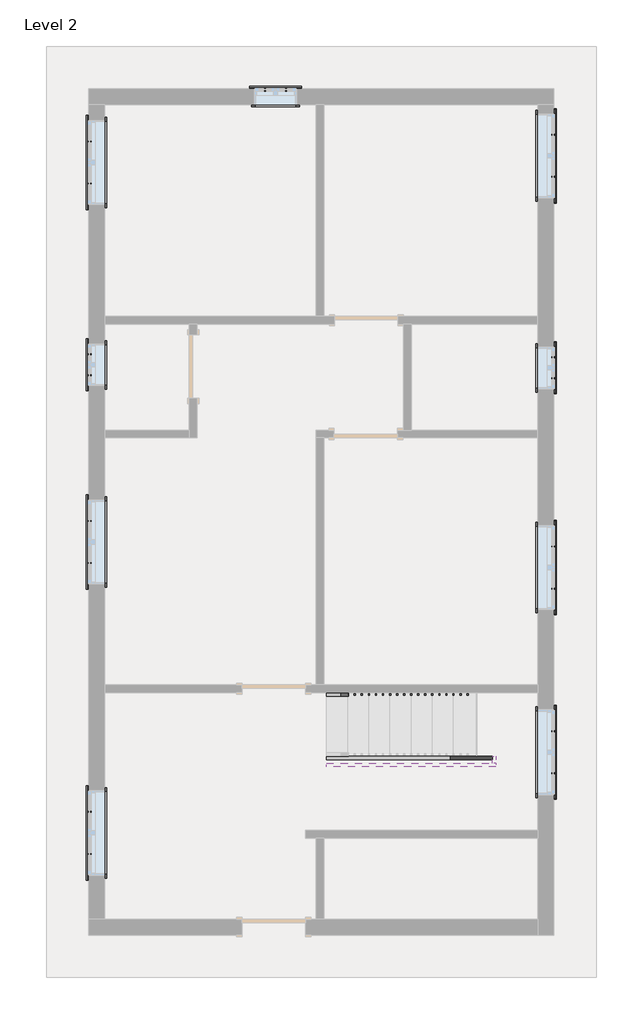
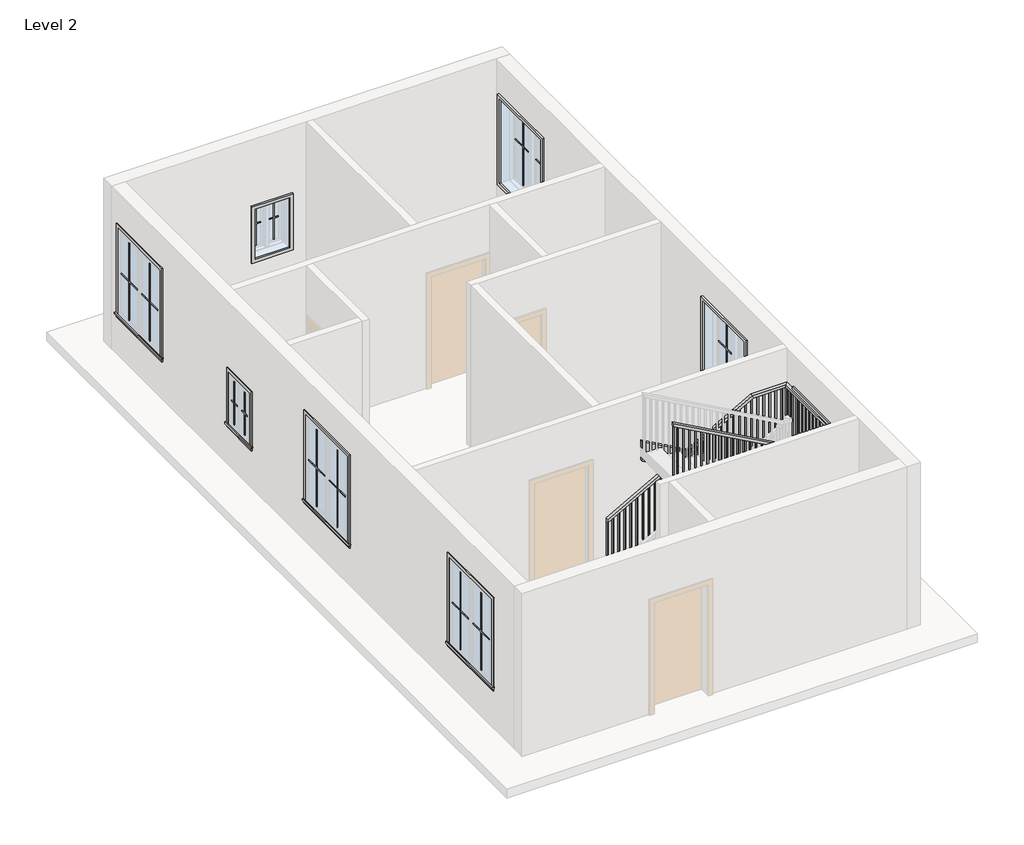
# One storey, part 2 of 2: 36 proxies, 3 members, 1 railing.
"""IFC4 building model written with IfcOpenShell, lengths in millimetres."""

from ifc_helpers import new_model, si_unit, frame, origin, place, context, project, spatial, polyline, outline, extrude, faceted_brep, transform, mapped, element, save
from components import muntin_pattern_2x2_muntin_pattern_2x2_6dad3731, muntin_pattern_2x2_muntin_pattern_2x2_a30a3345, muntin_pattern_2x2_muntin_pattern_2x2_53152e2c, muntin_pattern_2x2_muntin_pattern_2x2_e8f3e573, trim_window_exterior_flat_with_sill_92b9b949, trim_window_exterior_flat_with_sill_a665a915, trim_window_interior_flat_picture_frame_3bb882cf, trim_window_interior_flat_picture_frame_d485c387

model = new_model("IFC4")

# Units and contexts
model_context = context("Model", 3, world=origin())
ifc_project = project(units=[si_unit("LENGTHUNIT", "METRE", prefix="MILLI")], contexts=[model_context])

# Site, building, storey
site = spatial("IfcSite", under=ifc_project)
building = spatial("IfcBuilding", under=site)
storey = spatial("IfcBuildingStorey", under=building, Name="Level 2", Elevation=3048.0)

# Proxies
placement = place(None, origin())
muntin_pattern_2x2_muntin_pattern_2x2_shape = muntin_pattern_2x2_muntin_pattern_2x2_6dad3731(model_context)
element("IfcBuildingElementProxy", 1, Name="Muntin Pattern_2x2 : Muntin Pattern_2x2", ObjectType="Muntin Pattern_2x2 : Muntin Pattern_2x2", at=placement, inside=storey, context=model_context, shape_type="MappedRepresentation", body=[
    mapped(muntin_pattern_2x2_muntin_pattern_2x2_shape, transform((1279.525, 2947.4914062, 4032.25), x_axis=(0.0, 1.0, 0.0), y_axis=(-1.0, 0.0, 0.0), z_axis=(0.0, 0.0, 1.0))),
])
element("IfcBuildingElementProxy", 2, Name="Muntin Pattern_2x2 : Muntin Pattern_2x2", ObjectType="Muntin Pattern_2x2 : Muntin Pattern_2x2", at=placement, inside=storey, context=model_context, shape_type="MappedRepresentation", body=[
    mapped(muntin_pattern_2x2_muntin_pattern_2x2_shape, transform((1279.525, 7138.4914062, 4032.25), x_axis=(0.0, 1.0, 0.0), y_axis=(-1.0, 0.0, 0.0), z_axis=(0.0, 0.0, 1.0))),
])
element("IfcBuildingElementProxy", 3, Name="Muntin Pattern_2x2 : Muntin Pattern_2x2", ObjectType="Muntin Pattern_2x2 : Muntin Pattern_2x2", at=placement, inside=storey, context=model_context, shape_type="MappedRepresentation", body=[
    mapped(muntin_pattern_2x2_muntin_pattern_2x2_shape, transform((1279.525, 12605.8414062, 4032.25), x_axis=(0.0, 1.0, 0.0), y_axis=(-1.0, 0.0, 0.0), z_axis=(0.0, 0.0, 1.0))),
])
element("IfcBuildingElementProxy", 4, Name="Muntin Pattern_2x2 : Muntin Pattern_2x2", ObjectType="Muntin Pattern_2x2 : Muntin Pattern_2x2", at=placement, inside=storey, context=model_context, shape_type="MappedRepresentation", body=[
    mapped(muntin_pattern_2x2_muntin_pattern_2x2_shape, transform((7966.075, 13308.0125, 4032.25), x_axis=(0.0, -1.0, 0.0), y_axis=(1.0, 0.0, 0.0), z_axis=(0.0, 0.0, 1.0))),
])
element("IfcBuildingElementProxy", 5, Name="Muntin Pattern_2x2 : Muntin Pattern_2x2", ObjectType="Muntin Pattern_2x2 : Muntin Pattern_2x2", at=placement, inside=storey, context=model_context, shape_type="MappedRepresentation", body=[
    mapped(muntin_pattern_2x2_muntin_pattern_2x2_shape, transform((7966.075, 7377.1125, 4032.25), x_axis=(0.0, -1.0, 0.0), y_axis=(1.0, 0.0, 0.0), z_axis=(0.0, 0.0, 1.0))),
])
element("IfcBuildingElementProxy", 6, Name="Muntin Pattern_2x2 : Muntin Pattern_2x2", ObjectType="Muntin Pattern_2x2 : Muntin Pattern_2x2", at=placement, inside=storey, context=model_context, shape_type="MappedRepresentation", body=[
    mapped(muntin_pattern_2x2_muntin_pattern_2x2_shape, transform((7966.075, 4716.4625, 4032.25), x_axis=(0.0, -1.0, 0.0), y_axis=(1.0, 0.0, 0.0), z_axis=(0.0, 0.0, 1.0))),
])
muntin_pattern_2x2_muntin_pattern_2x2_2_shape = muntin_pattern_2x2_muntin_pattern_2x2_a30a3345(model_context)
element("IfcBuildingElementProxy", 7, Name="Muntin Pattern_2x2 : Muntin Pattern_2x2", ObjectType="Muntin Pattern_2x2 : Muntin Pattern_2x2", at=placement, inside=storey, context=model_context, shape_type="MappedRepresentation", body=[
    mapped(muntin_pattern_2x2_muntin_pattern_2x2_2_shape, transform((1279.525, 3553.9164063, 4032.25), x_axis=(0.0, -1.0, 0.0), y_axis=(1.0, 0.0, 0.0), z_axis=(0.0, 0.0, 1.0))),
])
element("IfcBuildingElementProxy", 8, Name="Muntin Pattern_2x2 : Muntin Pattern_2x2", ObjectType="Muntin Pattern_2x2 : Muntin Pattern_2x2", at=placement, inside=storey, context=model_context, shape_type="MappedRepresentation", body=[
    mapped(muntin_pattern_2x2_muntin_pattern_2x2_2_shape, transform((1279.525, 7744.9164062, 4032.25), x_axis=(0.0, -1.0, 0.0), y_axis=(1.0, 0.0, 0.0), z_axis=(0.0, 0.0, 1.0))),
])
element("IfcBuildingElementProxy", 9, Name="Muntin Pattern_2x2 : Muntin Pattern_2x2", ObjectType="Muntin Pattern_2x2 : Muntin Pattern_2x2", at=placement, inside=storey, context=model_context, shape_type="MappedRepresentation", body=[
    mapped(muntin_pattern_2x2_muntin_pattern_2x2_2_shape, transform((1279.525, 13212.2664062, 4032.25), x_axis=(0.0, -1.0, 0.0), y_axis=(1.0, 0.0, 0.0), z_axis=(0.0, 0.0, 1.0))),
])
element("IfcBuildingElementProxy", 10, Name="Muntin Pattern_2x2 : Muntin Pattern_2x2", ObjectType="Muntin Pattern_2x2 : Muntin Pattern_2x2", at=placement, inside=storey, context=model_context, shape_type="MappedRepresentation", body=[
    mapped(muntin_pattern_2x2_muntin_pattern_2x2_2_shape, transform((7966.075, 12701.5875, 4032.25), x_axis=(0.0, 1.0, 0.0), y_axis=(-1.0, 0.0, 0.0), z_axis=(0.0, 0.0, 1.0))),
])
element("IfcBuildingElementProxy", 11, Name="Muntin Pattern_2x2 : Muntin Pattern_2x2", ObjectType="Muntin Pattern_2x2 : Muntin Pattern_2x2", at=placement, inside=storey, context=model_context, shape_type="MappedRepresentation", body=[
    mapped(muntin_pattern_2x2_muntin_pattern_2x2_2_shape, transform((7966.075, 6770.6875, 4032.25), x_axis=(0.0, 1.0, 0.0), y_axis=(-1.0, 0.0, 0.0), z_axis=(0.0, 0.0, 1.0))),
])
element("IfcBuildingElementProxy", 12, Name="Muntin Pattern_2x2 : Muntin Pattern_2x2", ObjectType="Muntin Pattern_2x2 : Muntin Pattern_2x2", at=placement, inside=storey, context=model_context, shape_type="MappedRepresentation", body=[
    mapped(muntin_pattern_2x2_muntin_pattern_2x2_2_shape, transform((7966.075, 4110.0375, 4032.25), x_axis=(0.0, 1.0, 0.0), y_axis=(-1.0, 0.0, 0.0), z_axis=(0.0, 0.0, 1.0))),
])
muntin_pattern_2x2_muntin_pattern_2x2_3_shape = muntin_pattern_2x2_muntin_pattern_2x2_53152e2c(model_context)
element("IfcBuildingElementProxy", 13, Name="Muntin Pattern_2x2 : Muntin Pattern_2x2", ObjectType="Muntin Pattern_2x2 : Muntin Pattern_2x2", at=placement, inside=storey, context=model_context, shape_type="MappedRepresentation", body=[
    mapped(muntin_pattern_2x2_muntin_pattern_2x2_3_shape, transform((3811.5875, 13960.475, 4032.25), x_axis=(1.0, 0.0, 0.0), y_axis=(0.0, 1.0, 0.0), z_axis=(0.0, 0.0, 1.0))),
])
element("IfcBuildingElementProxy", 14, Name="Muntin Pattern_2x2 : Muntin Pattern_2x2", ObjectType="Muntin Pattern_2x2 : Muntin Pattern_2x2", at=placement, inside=storey, context=model_context, shape_type="MappedRepresentation", body=[
    mapped(muntin_pattern_2x2_muntin_pattern_2x2_3_shape, transform((7966.075, 10101.2625, 4032.25), x_axis=(0.0, -1.0, 0.0), y_axis=(1.0, 0.0, 0.0), z_axis=(0.0, 0.0, 1.0))),
])
element("IfcBuildingElementProxy", 15, Name="Muntin Pattern_2x2 : Muntin Pattern_2x2", ObjectType="Muntin Pattern_2x2 : Muntin Pattern_2x2", at=placement, inside=storey, context=model_context, shape_type="MappedRepresentation", body=[
    mapped(muntin_pattern_2x2_muntin_pattern_2x2_3_shape, transform((1279.525, 9843.5914062, 4032.25), x_axis=(0.0, 1.0, 0.0), y_axis=(-1.0, 0.0, 0.0), z_axis=(0.0, 0.0, 1.0))),
])
muntin_pattern_2x2_muntin_pattern_2x2_4_shape = muntin_pattern_2x2_muntin_pattern_2x2_e8f3e573(model_context)
element("IfcBuildingElementProxy", 16, Name="Muntin Pattern_2x2 : Muntin Pattern_2x2", ObjectType="Muntin Pattern_2x2 : Muntin Pattern_2x2", at=placement, inside=storey, context=model_context, shape_type="MappedRepresentation", body=[
    mapped(muntin_pattern_2x2_muntin_pattern_2x2_4_shape, transform((4113.2125, 13960.475, 4032.25), x_axis=(-1.0, 0.0, 0.0), y_axis=(0.0, -1.0, 0.0), z_axis=(0.0, 0.0, 1.0))),
])
element("IfcBuildingElementProxy", 17, Name="Muntin Pattern_2x2 : Muntin Pattern_2x2", ObjectType="Muntin Pattern_2x2 : Muntin Pattern_2x2", at=placement, inside=storey, context=model_context, shape_type="MappedRepresentation", body=[
    mapped(muntin_pattern_2x2_muntin_pattern_2x2_4_shape, transform((7966.075, 9799.6375, 4032.25), x_axis=(0.0, 1.0, 0.0), y_axis=(-1.0, 0.0, 0.0), z_axis=(0.0, 0.0, 1.0))),
])
element("IfcBuildingElementProxy", 18, Name="Muntin Pattern_2x2 : Muntin Pattern_2x2", ObjectType="Muntin Pattern_2x2 : Muntin Pattern_2x2", at=placement, inside=storey, context=model_context, shape_type="MappedRepresentation", body=[
    mapped(muntin_pattern_2x2_muntin_pattern_2x2_4_shape, transform((1279.525, 10145.2164062, 4032.25), x_axis=(0.0, -1.0, 0.0), y_axis=(1.0, 0.0, 0.0), z_axis=(0.0, 0.0, 1.0))),
])
trim_window_exterior_flat_with_sill_shape = trim_window_exterior_flat_with_sill_92b9b949(model_context)
element("IfcBuildingElementProxy", 19, Name="Trim-Window-Exterior-Flat : with Sill", ObjectType="Trim-Window-Exterior-Flat : with Sill", at=placement, inside=storey, context=model_context, shape_type="MappedRepresentation", body=[
    mapped(trim_window_exterior_flat_with_sill_shape, transform((1270.0, 3250.7039063, 5486.4), x_axis=(0.0, -1.0, 0.0), y_axis=(0.0, 0.0, 1.0), z_axis=(-1.0, 0.0, 0.0))),
])
element("IfcBuildingElementProxy", 20, Name="Trim-Window-Exterior-Flat : with Sill", ObjectType="Trim-Window-Exterior-Flat : with Sill", at=placement, inside=storey, context=model_context, shape_type="MappedRepresentation", body=[
    mapped(trim_window_exterior_flat_with_sill_shape, transform((1270.0, 7441.7039063, 5486.4), x_axis=(0.0, -1.0, 0.0), y_axis=(0.0, 0.0, 1.0), z_axis=(-1.0, 0.0, 0.0))),
])
element("IfcBuildingElementProxy", 21, Name="Trim-Window-Exterior-Flat : with Sill", ObjectType="Trim-Window-Exterior-Flat : with Sill", at=placement, inside=storey, context=model_context, shape_type="MappedRepresentation", body=[
    mapped(trim_window_exterior_flat_with_sill_shape, transform((1270.0, 12909.0539063, 5486.4), x_axis=(0.0, -1.0, 0.0), y_axis=(0.0, 0.0, 1.0), z_axis=(-1.0, 0.0, 0.0))),
])
element("IfcBuildingElementProxy", 22, Name="Trim-Window-Exterior-Flat : with Sill", ObjectType="Trim-Window-Exterior-Flat : with Sill", at=placement, inside=storey, context=model_context, shape_type="MappedRepresentation", body=[
    mapped(trim_window_exterior_flat_with_sill_shape, transform((7975.6, 13004.8, 5486.4), x_axis=(0.0, 1.0, 0.0), y_axis=(0.0, 0.0, 1.0), z_axis=(1.0, 0.0, 0.0))),
])
element("IfcBuildingElementProxy", 23, Name="Trim-Window-Exterior-Flat : with Sill", ObjectType="Trim-Window-Exterior-Flat : with Sill", at=placement, inside=storey, context=model_context, shape_type="MappedRepresentation", body=[
    mapped(trim_window_exterior_flat_with_sill_shape, transform((7975.6, 7073.9, 5486.4), x_axis=(0.0, 1.0, 0.0), y_axis=(0.0, 0.0, 1.0), z_axis=(1.0, 0.0, 0.0))),
])
element("IfcBuildingElementProxy", 24, Name="Trim-Window-Exterior-Flat : with Sill", ObjectType="Trim-Window-Exterior-Flat : with Sill", at=placement, inside=storey, context=model_context, shape_type="MappedRepresentation", body=[
    mapped(trim_window_exterior_flat_with_sill_shape, transform((7975.6, 4413.25, 5486.4), x_axis=(0.0, 1.0, 0.0), y_axis=(0.0, 0.0, 1.0), z_axis=(1.0, 0.0, 0.0))),
])
trim_window_exterior_flat_with_sill_2_shape = trim_window_exterior_flat_with_sill_a665a915(model_context)
element("IfcBuildingElementProxy", 25, Name="Trim-Window-Exterior-Flat : with Sill", ObjectType="Trim-Window-Exterior-Flat : with Sill", at=placement, inside=storey, context=model_context, shape_type="MappedRepresentation", body=[
    mapped(trim_window_exterior_flat_with_sill_2_shape, transform((3962.4, 13970.0, 4876.8), x_axis=(-1.0, 0.0, 0.0), y_axis=(0.0, 0.0, 1.0), z_axis=(0.0, 1.0, 0.0))),
])
element("IfcBuildingElementProxy", 26, Name="Trim-Window-Exterior-Flat : with Sill", ObjectType="Trim-Window-Exterior-Flat : with Sill", at=placement, inside=storey, context=model_context, shape_type="MappedRepresentation", body=[
    mapped(trim_window_exterior_flat_with_sill_2_shape, transform((7975.6, 9950.45, 4876.8), x_axis=(0.0, 1.0, 0.0), y_axis=(0.0, 0.0, 1.0), z_axis=(1.0, 0.0, 0.0))),
])
element("IfcBuildingElementProxy", 27, Name="Trim-Window-Exterior-Flat : with Sill", ObjectType="Trim-Window-Exterior-Flat : with Sill", at=placement, inside=storey, context=model_context, shape_type="MappedRepresentation", body=[
    mapped(trim_window_exterior_flat_with_sill_2_shape, transform((1270.0, 9994.4039062, 4876.8), x_axis=(0.0, -1.0, 0.0), y_axis=(0.0, 0.0, 1.0), z_axis=(-1.0, 0.0, 0.0))),
])
trim_window_interior_flat_picture_frame_shape = trim_window_interior_flat_picture_frame_3bb882cf(model_context)
element("IfcBuildingElementProxy", 28, Name="Trim-Window-Interior-Flat : Picture Frame", ObjectType="Trim-Window-Interior-Flat : Picture Frame", at=placement, inside=storey, context=model_context, shape_type="MappedRepresentation", body=[
    mapped(trim_window_interior_flat_picture_frame_shape, transform((1498.6, 3250.7039063, 5486.4), x_axis=(0.0, 1.0, 0.0), y_axis=(0.0, 0.0, 1.0), z_axis=(1.0, 0.0, 0.0))),
])
element("IfcBuildingElementProxy", 29, Name="Trim-Window-Interior-Flat : Picture Frame", ObjectType="Trim-Window-Interior-Flat : Picture Frame", at=placement, inside=storey, context=model_context, shape_type="MappedRepresentation", body=[
    mapped(trim_window_interior_flat_picture_frame_shape, transform((1498.6, 7441.7039062, 5486.4), x_axis=(0.0, 1.0, 0.0), y_axis=(0.0, 0.0, 1.0), z_axis=(1.0, 0.0, 0.0))),
])
element("IfcBuildingElementProxy", 30, Name="Trim-Window-Interior-Flat : Picture Frame", ObjectType="Trim-Window-Interior-Flat : Picture Frame", at=placement, inside=storey, context=model_context, shape_type="MappedRepresentation", body=[
    mapped(trim_window_interior_flat_picture_frame_shape, transform((1498.6, 12909.0539062, 5486.4), x_axis=(0.0, 1.0, 0.0), y_axis=(0.0, 0.0, 1.0), z_axis=(1.0, 0.0, 0.0))),
])
element("IfcBuildingElementProxy", 31, Name="Trim-Window-Interior-Flat : Picture Frame", ObjectType="Trim-Window-Interior-Flat : Picture Frame", at=placement, inside=storey, context=model_context, shape_type="MappedRepresentation", body=[
    mapped(trim_window_interior_flat_picture_frame_shape, transform((7747.0, 13004.8, 5486.4), x_axis=(0.0, -1.0, 0.0), y_axis=(0.0, 0.0, 1.0), z_axis=(-1.0, 0.0, 0.0))),
])
element("IfcBuildingElementProxy", 32, Name="Trim-Window-Interior-Flat : Picture Frame", ObjectType="Trim-Window-Interior-Flat : Picture Frame", at=placement, inside=storey, context=model_context, shape_type="MappedRepresentation", body=[
    mapped(trim_window_interior_flat_picture_frame_shape, transform((7747.0, 7073.9, 5486.4), x_axis=(0.0, -1.0, 0.0), y_axis=(0.0, 0.0, 1.0), z_axis=(-1.0, 0.0, 0.0))),
])
element("IfcBuildingElementProxy", 33, Name="Trim-Window-Interior-Flat : Picture Frame", ObjectType="Trim-Window-Interior-Flat : Picture Frame", at=placement, inside=storey, context=model_context, shape_type="MappedRepresentation", body=[
    mapped(trim_window_interior_flat_picture_frame_shape, transform((7747.0, 4413.25, 5486.4), x_axis=(0.0, -1.0, 0.0), y_axis=(0.0, 0.0, 1.0), z_axis=(-1.0, 0.0, 0.0))),
])
trim_window_interior_flat_picture_frame_2_shape = trim_window_interior_flat_picture_frame_d485c387(model_context)
element("IfcBuildingElementProxy", 34, Name="Trim-Window-Interior-Flat : Picture Frame", ObjectType="Trim-Window-Interior-Flat : Picture Frame", at=placement, inside=storey, context=model_context, shape_type="MappedRepresentation", body=[
    mapped(trim_window_interior_flat_picture_frame_2_shape, transform((3962.4, 13741.4, 4876.8), x_axis=(1.0, 0.0, 0.0), y_axis=(0.0, 0.0, 1.0), z_axis=(0.0, -1.0, 0.0))),
])
element("IfcBuildingElementProxy", 35, Name="Trim-Window-Interior-Flat : Picture Frame", ObjectType="Trim-Window-Interior-Flat : Picture Frame", at=placement, inside=storey, context=model_context, shape_type="MappedRepresentation", body=[
    mapped(trim_window_interior_flat_picture_frame_2_shape, transform((7747.0, 9950.45, 4876.8), x_axis=(0.0, -1.0, 0.0), y_axis=(0.0, 0.0, 1.0), z_axis=(-1.0, 0.0, 0.0))),
])
element("IfcBuildingElementProxy", 36, Name="Trim-Window-Interior-Flat : Picture Frame", ObjectType="Trim-Window-Interior-Flat : Picture Frame", at=placement, inside=storey, context=model_context, shape_type="MappedRepresentation", body=[
    mapped(trim_window_interior_flat_picture_frame_2_shape, transform((1498.6, 9994.4039062, 4876.8), x_axis=(0.0, 1.0, 0.0), y_axis=(0.0, 0.0, 1.0), z_axis=(1.0, 0.0, 0.0))),
])

# Members
element("IfcMember", 37, ObjectType="Stringer - 2\" Width", at=placement, inside=storey, context=model_context, shape_type="SweptSolid", body=[
    extrude(outline(polyline([(3255.5983948, 4699.0), (3048.0, 4699.0), (3048.0, 4952.9445028), (4233.3641651, 7086.6), (4582.0428392, 7086.6), (3255.5983948, 4699.0)])), frame((0.0, 4305.3, 0.0), z_axis=(0.0, 1.0, 0.0), x_axis=(0.0, 0.0, 1.0)), (0.0, 0.0, 1.0), 50.8),
])
element("IfcMember", 38, ObjectType="Stringer - 2\" Width", at=placement, inside=storey, context=model_context, shape_type="SweptSolid", body=[
    extrude(outline(polyline([(7086.6, 4356.1), (7137.4, 4356.1), (7137.4, 4254.5), (7086.6, 4254.5), (7086.6, 4356.1)])), frame((0.0, 0.0, 4343.4), z_axis=(0.0, 0.0, 1.0), x_axis=(1.0, 0.0, 0.0)), (0.0, 0.0, 1.0), 304.8),
])
element("IfcMember", 39, ObjectType="Stringer - 2\" Width", at=placement, inside=storey, context=model_context, shape_type="SweptSolid", body=[
    extrude(outline(polyline([(4430.9197207, 7137.4), (4779.5983948, 7137.4), (6134.2650614, 4699.0), (5785.5863873, 4699.0), (4430.9197207, 7137.4)])), frame((0.0, 4203.7, 0.0), z_axis=(0.0, 1.0, 0.0), x_axis=(0.0, 0.0, 1.0)), (0.0, 0.0, 1.0), 50.8),
])

# Railing
element("IfcRailing", 40, ObjectType="Handrail - Rectangular", at=placement, inside=storey, context=model_context, shape_type="SolidModel", body=[
    faceted_brep([(4699.0, 5270.5, 4131.7333333), (4699.0, 5270.5, 4073.620221), (4699.0, 5219.7, 4073.620221), (4699.0, 5219.7, 4131.7333333), (7137.4, 5270.5, 5486.4), (7150.5636022, 5270.5, 5435.6), (7150.5636022, 5219.7, 5435.6), (7137.4, 5219.7, 5486.4), (7747.0, 5270.5, 5486.4), (7747.0, 5270.5, 5435.6), (7696.2, 5219.7, 5435.6), (7696.2, 5219.7, 5486.4), (7747.0, 3289.3, 5486.4), (7747.0, 3289.3, 5435.6), (7696.2, 3340.1, 5435.6), (7696.2, 3340.1, 5486.4), (7442.2, 3289.3, 5486.4), (7429.0363978, 3289.3, 5435.6), (7429.0363978, 3340.1, 5435.6), (7442.2, 3340.1, 5486.4), (4699.0, 3289.3, 7010.4), (4699.0, 3340.1, 7010.4), (4699.0, 3340.1, 6952.2868876), (4699.0, 3289.3, 6952.2868876)], [[[0, 1, 2, 3]], [[1, 0, 4, 5]], [[2, 1, 5, 6]], [[3, 2, 6, 7]], [[0, 3, 7, 4]], [[5, 4, 8, 9]], [[6, 5, 9, 10]], [[7, 6, 10, 11]], [[4, 7, 11, 8]], [[9, 8, 12, 13]], [[10, 9, 13, 14]], [[11, 10, 14, 15]], [[8, 11, 15, 12]], [[13, 12, 16, 17]], [[14, 13, 17, 18]], [[15, 14, 18, 19]], [[12, 15, 19, 16]], [[20, 21, 22, 23]], [[17, 16, 20, 23]], [[18, 17, 23, 22]], [[19, 18, 22, 21]], [[16, 19, 21, 20]]]),
    extrude(outline(polyline([(6915.245221, 4765.675), (5926.6666667, 4765.675), (5926.6666667, 4784.725), (6904.6618876, 4784.725), (6915.245221, 4765.675)])), frame((0.0, 3305.175, 0.0), z_axis=(0.0, 1.0, 0.0), x_axis=(0.0, 0.0, 1.0)), (0.0, 0.0, 1.0), 19.05),
    extrude(outline(polyline([(6858.8007765, 4867.275), (5926.6666667, 4867.275), (5926.6666667, 4886.325), (6848.2174432, 4886.325), (6858.8007765, 4867.275)])), frame((0.0, 3305.175, 0.0), z_axis=(0.0, 1.0, 0.0), x_axis=(0.0, 0.0, 1.0)), (0.0, 0.0, 1.0), 19.05),
    extrude(outline(polyline([(6802.3563321, 4968.875), (5926.6666667, 4968.875), (5926.6666667, 4987.925), (6791.7729988, 4987.925), (6802.3563321, 4968.875)])), frame((0.0, 3305.175, 0.0), z_axis=(0.0, 1.0, 0.0), x_axis=(0.0, 0.0, 1.0)), (0.0, 0.0, 1.0), 19.05),
    extrude(outline(polyline([(6745.9118876, 5070.475), (5757.3333333, 5070.475), (5757.3333333, 5089.525), (6735.3285543, 5089.525), (6745.9118876, 5070.475)])), frame((0.0, 3305.175, 0.0), z_axis=(0.0, 1.0, 0.0), x_axis=(0.0, 0.0, 1.0)), (0.0, 0.0, 1.0), 19.05),
    extrude(outline(polyline([(6689.4674432, 5172.075), (5757.3333333, 5172.075), (5757.3333333, 5191.125), (6678.8841099, 5191.125), (6689.4674432, 5172.075)])), frame((0.0, 3305.175, 0.0), z_axis=(0.0, 1.0, 0.0), x_axis=(0.0, 0.0, 1.0)), (0.0, 0.0, 1.0), 19.05),
    extrude(outline(polyline([(6633.0229988, 5273.675), (5757.3333333, 5273.675), (5757.3333333, 5292.725), (6622.4396654, 5292.725), (6633.0229988, 5273.675)])), frame((0.0, 3305.175, 0.0), z_axis=(0.0, 1.0, 0.0), x_axis=(0.0, 0.0, 1.0)), (0.0, 0.0, 1.0), 19.05),
    extrude(outline(polyline([(6576.5785543, 5375.275), (5588.0, 5375.275), (5588.0, 5394.325), (6565.995221, 5394.325), (6576.5785543, 5375.275)])), frame((0.0, 3305.175, 0.0), z_axis=(0.0, 1.0, 0.0), x_axis=(0.0, 0.0, 1.0)), (0.0, 0.0, 1.0), 19.05),
    extrude(outline(polyline([(6520.1341099, 5476.875), (5588.0, 5476.875), (5588.0, 5495.925), (6509.5507765, 5495.925), (6520.1341099, 5476.875)])), frame((0.0, 3305.175, 0.0), z_axis=(0.0, 1.0, 0.0), x_axis=(0.0, 0.0, 1.0)), (0.0, 0.0, 1.0), 19.05),
    extrude(outline(polyline([(6463.6896654, 5578.475), (5588.0, 5578.475), (5588.0, 5597.525), (6453.1063321, 5597.525), (6463.6896654, 5578.475)])), frame((0.0, 3305.175, 0.0), z_axis=(0.0, 1.0, 0.0), x_axis=(0.0, 0.0, 1.0)), (0.0, 0.0, 1.0), 19.05),
    extrude(outline(polyline([(6407.245221, 5680.075), (5418.6666667, 5680.075), (5418.6666667, 5699.125), (6396.6618876, 5699.125), (6407.245221, 5680.075)])), frame((0.0, 3305.175, 0.0), z_axis=(0.0, 1.0, 0.0), x_axis=(0.0, 0.0, 1.0)), (0.0, 0.0, 1.0), 19.05),
    extrude(outline(polyline([(6350.8007765, 5781.675), (5418.6666667, 5781.675), (5418.6666667, 5800.725), (6340.2174432, 5800.725), (6350.8007765, 5781.675)])), frame((0.0, 3305.175, 0.0), z_axis=(0.0, 1.0, 0.0), x_axis=(0.0, 0.0, 1.0)), (0.0, 0.0, 1.0), 19.05),
    extrude(outline(polyline([(6294.3563321, 5883.275), (5418.6666667, 5883.275), (5418.6666667, 5902.325), (6283.7729988, 5902.325), (6294.3563321, 5883.275)])), frame((0.0, 3305.175, 0.0), z_axis=(0.0, 1.0, 0.0), x_axis=(0.0, 0.0, 1.0)), (0.0, 0.0, 1.0), 19.05),
    extrude(outline(polyline([(6237.9118876, 5984.875), (5249.3333333, 5984.875), (5249.3333333, 6003.925), (6227.3285543, 6003.925), (6237.9118876, 5984.875)])), frame((0.0, 3305.175, 0.0), z_axis=(0.0, 1.0, 0.0), x_axis=(0.0, 0.0, 1.0)), (0.0, 0.0, 1.0), 19.05),
    extrude(outline(polyline([(6181.4674432, 6086.475), (5249.3333333, 6086.475), (5249.3333333, 6105.525), (6170.8841099, 6105.525), (6181.4674432, 6086.475)])), frame((0.0, 3305.175, 0.0), z_axis=(0.0, 1.0, 0.0), x_axis=(0.0, 0.0, 1.0)), (0.0, 0.0, 1.0), 19.05),
    extrude(outline(polyline([(6125.0229988, 6188.075), (5249.3333333, 6188.075), (5249.3333333, 6207.125), (6114.4396654, 6207.125), (6125.0229988, 6188.075)])), frame((0.0, 3305.175, 0.0), z_axis=(0.0, 1.0, 0.0), x_axis=(0.0, 0.0, 1.0)), (0.0, 0.0, 1.0), 19.05),
    extrude(outline(polyline([(6068.5785543, 6289.675), (5080.0, 6289.675), (5080.0, 6308.725), (6057.995221, 6308.725), (6068.5785543, 6289.675)])), frame((0.0, 3305.175, 0.0), z_axis=(0.0, 1.0, 0.0), x_axis=(0.0, 0.0, 1.0)), (0.0, 0.0, 1.0), 19.05),
    extrude(outline(polyline([(6012.1341099, 6391.275), (5080.0, 6391.275), (5080.0, 6410.325), (6001.5507765, 6410.325), (6012.1341099, 6391.275)])), frame((0.0, 3305.175, 0.0), z_axis=(0.0, 1.0, 0.0), x_axis=(0.0, 0.0, 1.0)), (0.0, 0.0, 1.0), 19.05),
    extrude(outline(polyline([(5955.6896654, 6492.875), (5080.0, 6492.875), (5080.0, 6511.925), (5945.1063321, 6511.925), (5955.6896654, 6492.875)])), frame((0.0, 3305.175, 0.0), z_axis=(0.0, 1.0, 0.0), x_axis=(0.0, 0.0, 1.0)), (0.0, 0.0, 1.0), 19.05),
    extrude(outline(polyline([(5899.245221, 6594.475), (4910.6666667, 6594.475), (4910.6666667, 6613.525), (5888.6618876, 6613.525), (5899.245221, 6594.475)])), frame((0.0, 3305.175, 0.0), z_axis=(0.0, 1.0, 0.0), x_axis=(0.0, 0.0, 1.0)), (0.0, 0.0, 1.0), 19.05),
    extrude(outline(polyline([(5842.8007765, 6696.075), (4910.6666667, 6696.075), (4910.6666667, 6715.125), (5832.2174432, 6715.125), (5842.8007765, 6696.075)])), frame((0.0, 3305.175, 0.0), z_axis=(0.0, 1.0, 0.0), x_axis=(0.0, 0.0, 1.0)), (0.0, 0.0, 1.0), 19.05),
    extrude(outline(polyline([(5786.3563321, 6797.675), (4910.6666667, 6797.675), (4910.6666667, 6816.725), (5775.7729988, 6816.725), (5786.3563321, 6797.675)])), frame((0.0, 3305.175, 0.0), z_axis=(0.0, 1.0, 0.0), x_axis=(0.0, 0.0, 1.0)), (0.0, 0.0, 1.0), 19.05),
    extrude(outline(polyline([(5729.9118876, 6899.275), (4741.3333333, 6899.275), (4741.3333333, 6918.325), (5719.3285543, 6918.325), (5729.9118876, 6899.275)])), frame((0.0, 3305.175, 0.0), z_axis=(0.0, 1.0, 0.0), x_axis=(0.0, 0.0, 1.0)), (0.0, 0.0, 1.0), 19.05),
    extrude(outline(polyline([(5673.4674432, 7000.875), (4741.3333333, 7000.875), (4741.3333333, 7019.925), (5662.8841099, 7019.925), (5673.4674432, 7000.875)])), frame((0.0, 3305.175, 0.0), z_axis=(0.0, 1.0, 0.0), x_axis=(0.0, 0.0, 1.0)), (0.0, 0.0, 1.0), 19.05),
    extrude(outline(polyline([(5617.0229988, 7102.475), (4741.3333333, 7102.475), (4741.3333333, 7121.525), (5606.4396654, 7121.525), (5617.0229988, 7102.475)])), frame((0.0, 3305.175, 0.0), z_axis=(0.0, 1.0, 0.0), x_axis=(0.0, 0.0, 1.0)), (0.0, 0.0, 1.0), 19.05),
    extrude(outline(polyline([(5560.5785543, 7204.075), (4572.0, 7204.075), (4572.0, 7223.125), (5549.995221, 7223.125), (5560.5785543, 7204.075)])), frame((0.0, 3305.175, 0.0), z_axis=(0.0, 1.0, 0.0), x_axis=(0.0, 0.0, 1.0)), (0.0, 0.0, 1.0), 19.05),
    extrude(outline(polyline([(5504.1341099, 7305.675), (4572.0, 7305.675), (4572.0, 7324.725), (5493.5507765, 7324.725), (5504.1341099, 7305.675)])), frame((0.0, 3305.175, 0.0), z_axis=(0.0, 1.0, 0.0), x_axis=(0.0, 0.0, 1.0)), (0.0, 0.0, 1.0), 19.05),
    extrude(outline(polyline([(5447.6896654, 7407.275), (4572.0, 7407.275), (4572.0, 7426.325), (5437.1063321, 7426.325), (5447.6896654, 7407.275)])), frame((0.0, 3305.175, 0.0), z_axis=(0.0, 1.0, 0.0), x_axis=(0.0, 0.0, 1.0)), (0.0, 0.0, 1.0), 19.05),
    extrude(outline(polyline([(7527.925, 3305.175), (7508.875, 3305.175), (7508.875, 3324.225), (7527.925, 3324.225), (7527.925, 3305.175)])), frame((0.0, 0.0, 4572.0), z_axis=(0.0, 0.0, 1.0), x_axis=(1.0, 0.0, 0.0)), (0.0, 0.0, 1.0), 863.6),
    extrude(outline(polyline([(7629.525, 3305.175), (7610.475, 3305.175), (7610.475, 3324.225), (7629.525, 3324.225), (7629.525, 3305.175)])), frame((0.0, 0.0, 4572.0), z_axis=(0.0, 0.0, 1.0), x_axis=(1.0, 0.0, 0.0)), (0.0, 0.0, 1.0), 863.6),
    extrude(outline(polyline([(7731.125, 3425.825), (7731.125, 3406.775), (7712.075, 3406.775), (7712.075, 3425.825), (7731.125, 3425.825)])), frame((0.0, 0.0, 4572.0), z_axis=(0.0, 0.0, 1.0), x_axis=(1.0, 0.0, 0.0)), (0.0, 0.0, 1.0), 863.6),
    extrude(outline(polyline([(7731.125, 3527.425), (7731.125, 3508.375), (7712.075, 3508.375), (7712.075, 3527.425), (7731.125, 3527.425)])), frame((0.0, 0.0, 4572.0), z_axis=(0.0, 0.0, 1.0), x_axis=(1.0, 0.0, 0.0)), (0.0, 0.0, 1.0), 863.6),
    extrude(outline(polyline([(7731.125, 3629.025), (7731.125, 3609.975), (7712.075, 3609.975), (7712.075, 3629.025), (7731.125, 3629.025)])), frame((0.0, 0.0, 4572.0), z_axis=(0.0, 0.0, 1.0), x_axis=(1.0, 0.0, 0.0)), (0.0, 0.0, 1.0), 863.6),
    extrude(outline(polyline([(7731.125, 3730.625), (7731.125, 3711.575), (7712.075, 3711.575), (7712.075, 3730.625), (7731.125, 3730.625)])), frame((0.0, 0.0, 4572.0), z_axis=(0.0, 0.0, 1.0), x_axis=(1.0, 0.0, 0.0)), (0.0, 0.0, 1.0), 863.6),
    extrude(outline(polyline([(7731.125, 3832.225), (7731.125, 3813.175), (7712.075, 3813.175), (7712.075, 3832.225), (7731.125, 3832.225)])), frame((0.0, 0.0, 4572.0), z_axis=(0.0, 0.0, 1.0), x_axis=(1.0, 0.0, 0.0)), (0.0, 0.0, 1.0), 863.6),
    extrude(outline(polyline([(7731.125, 3933.825), (7731.125, 3914.775), (7712.075, 3914.775), (7712.075, 3933.825), (7731.125, 3933.825)])), frame((0.0, 0.0, 4572.0), z_axis=(0.0, 0.0, 1.0), x_axis=(1.0, 0.0, 0.0)), (0.0, 0.0, 1.0), 863.6),
    extrude(outline(polyline([(7731.125, 4035.425), (7731.125, 4016.375), (7712.075, 4016.375), (7712.075, 4035.425), (7731.125, 4035.425)])), frame((0.0, 0.0, 4572.0), z_axis=(0.0, 0.0, 1.0), x_axis=(1.0, 0.0, 0.0)), (0.0, 0.0, 1.0), 863.6),
    extrude(outline(polyline([(7731.125, 4137.025), (7731.125, 4117.975), (7712.075, 4117.975), (7712.075, 4137.025), (7731.125, 4137.025)])), frame((0.0, 0.0, 4572.0), z_axis=(0.0, 0.0, 1.0), x_axis=(1.0, 0.0, 0.0)), (0.0, 0.0, 1.0), 863.6),
    extrude(outline(polyline([(7731.125, 4238.625), (7731.125, 4219.575), (7712.075, 4219.575), (7712.075, 4238.625), (7731.125, 4238.625)])), frame((0.0, 0.0, 4572.0), z_axis=(0.0, 0.0, 1.0), x_axis=(1.0, 0.0, 0.0)), (0.0, 0.0, 1.0), 863.6),
    extrude(outline(polyline([(7731.125, 4340.225), (7731.125, 4321.175), (7712.075, 4321.175), (7712.075, 4340.225), (7731.125, 4340.225)])), frame((0.0, 0.0, 4572.0), z_axis=(0.0, 0.0, 1.0), x_axis=(1.0, 0.0, 0.0)), (0.0, 0.0, 1.0), 863.6),
    extrude(outline(polyline([(7731.125, 4441.825), (7731.125, 4422.775), (7712.075, 4422.775), (7712.075, 4441.825), (7731.125, 4441.825)])), frame((0.0, 0.0, 4572.0), z_axis=(0.0, 0.0, 1.0), x_axis=(1.0, 0.0, 0.0)), (0.0, 0.0, 1.0), 863.6),
    extrude(outline(polyline([(7731.125, 4543.425), (7731.125, 4524.375), (7712.075, 4524.375), (7712.075, 4543.425), (7731.125, 4543.425)])), frame((0.0, 0.0, 4572.0), z_axis=(0.0, 0.0, 1.0), x_axis=(1.0, 0.0, 0.0)), (0.0, 0.0, 1.0), 863.6),
    extrude(outline(polyline([(7731.125, 4645.025), (7731.125, 4625.975), (7712.075, 4625.975), (7712.075, 4645.025), (7731.125, 4645.025)])), frame((0.0, 0.0, 4572.0), z_axis=(0.0, 0.0, 1.0), x_axis=(1.0, 0.0, 0.0)), (0.0, 0.0, 1.0), 863.6),
    extrude(outline(polyline([(7731.125, 4746.625), (7731.125, 4727.575), (7712.075, 4727.575), (7712.075, 4746.625), (7731.125, 4746.625)])), frame((0.0, 0.0, 4572.0), z_axis=(0.0, 0.0, 1.0), x_axis=(1.0, 0.0, 0.0)), (0.0, 0.0, 1.0), 863.6),
    extrude(outline(polyline([(7731.125, 4848.225), (7731.125, 4829.175), (7712.075, 4829.175), (7712.075, 4848.225), (7731.125, 4848.225)])), frame((0.0, 0.0, 4572.0), z_axis=(0.0, 0.0, 1.0), x_axis=(1.0, 0.0, 0.0)), (0.0, 0.0, 1.0), 863.6),
    extrude(outline(polyline([(7731.125, 4949.825), (7731.125, 4930.775), (7712.075, 4930.775), (7712.075, 4949.825), (7731.125, 4949.825)])), frame((0.0, 0.0, 4572.0), z_axis=(0.0, 0.0, 1.0), x_axis=(1.0, 0.0, 0.0)), (0.0, 0.0, 1.0), 863.6),
    extrude(outline(polyline([(7731.125, 5051.425), (7731.125, 5032.375), (7712.075, 5032.375), (7712.075, 5051.425), (7731.125, 5051.425)])), frame((0.0, 0.0, 4572.0), z_axis=(0.0, 0.0, 1.0), x_axis=(1.0, 0.0, 0.0)), (0.0, 0.0, 1.0), 863.6),
    extrude(outline(polyline([(7731.125, 5153.025), (7731.125, 5133.975), (7712.075, 5133.975), (7712.075, 5153.025), (7731.125, 5153.025)])), frame((0.0, 0.0, 4572.0), z_axis=(0.0, 0.0, 1.0), x_axis=(1.0, 0.0, 0.0)), (0.0, 0.0, 1.0), 863.6),
    extrude(outline(polyline([(7635.875, 5254.625), (7654.925, 5254.625), (7654.925, 5235.575), (7635.875, 5235.575), (7635.875, 5254.625)])), frame((0.0, 0.0, 4572.0), z_axis=(0.0, 0.0, 1.0), x_axis=(1.0, 0.0, 0.0)), (0.0, 0.0, 1.0), 863.6),
    extrude(outline(polyline([(7534.275, 5254.625), (7553.325, 5254.625), (7553.325, 5235.575), (7534.275, 5235.575), (7534.275, 5254.625)])), frame((0.0, 0.0, 4572.0), z_axis=(0.0, 0.0, 1.0), x_axis=(1.0, 0.0, 0.0)), (0.0, 0.0, 1.0), 863.6),
    extrude(outline(polyline([(7432.675, 5254.625), (7451.725, 5254.625), (7451.725, 5235.575), (7432.675, 5235.575), (7432.675, 5254.625)])), frame((0.0, 0.0, 4572.0), z_axis=(0.0, 0.0, 1.0), x_axis=(1.0, 0.0, 0.0)), (0.0, 0.0, 1.0), 863.6),
    extrude(outline(polyline([(7331.075, 5254.625), (7350.125, 5254.625), (7350.125, 5235.575), (7331.075, 5235.575), (7331.075, 5254.625)])), frame((0.0, 0.0, 4572.0), z_axis=(0.0, 0.0, 1.0), x_axis=(1.0, 0.0, 0.0)), (0.0, 0.0, 1.0), 863.6),
    extrude(outline(polyline([(7229.475, 5254.625), (7248.525, 5254.625), (7248.525, 5235.575), (7229.475, 5235.575), (7229.475, 5254.625)])), frame((0.0, 0.0, 4572.0), z_axis=(0.0, 0.0, 1.0), x_axis=(1.0, 0.0, 0.0)), (0.0, 0.0, 1.0), 863.6),
    extrude(outline(polyline([(5422.995221, 7127.875), (4572.0, 7127.875), (4572.0, 7146.925), (5433.5785543, 7146.925), (5422.995221, 7127.875)])), frame((0.0, 5235.575, 0.0), z_axis=(0.0, 1.0, 0.0), x_axis=(0.0, 0.0, 1.0)), (0.0, 0.0, 1.0), 19.05),
    extrude(outline(polyline([(5366.5507765, 7026.275), (4402.6666667, 7026.275), (4402.6666667, 7045.325), (5377.1341099, 7045.325), (5366.5507765, 7026.275)])), frame((0.0, 5235.575, 0.0), z_axis=(0.0, 1.0, 0.0), x_axis=(0.0, 0.0, 1.0)), (0.0, 0.0, 1.0), 19.05),
    extrude(outline(polyline([(5310.1063321, 6924.675), (4402.6666667, 6924.675), (4402.6666667, 6943.725), (5320.6896654, 6943.725), (5310.1063321, 6924.675)])), frame((0.0, 5235.575, 0.0), z_axis=(0.0, 1.0, 0.0), x_axis=(0.0, 0.0, 1.0)), (0.0, 0.0, 1.0), 19.05),
    extrude(outline(polyline([(5253.6618876, 6823.075), (4402.6666667, 6823.075), (4402.6666667, 6842.125), (5264.245221, 6842.125), (5253.6618876, 6823.075)])), frame((0.0, 5235.575, 0.0), z_axis=(0.0, 1.0, 0.0), x_axis=(0.0, 0.0, 1.0)), (0.0, 0.0, 1.0), 19.05),
    extrude(outline(polyline([(5197.2174432, 6721.475), (4233.3333333, 6721.475), (4233.3333333, 6740.525), (5207.8007765, 6740.525), (5197.2174432, 6721.475)])), frame((0.0, 5235.575, 0.0), z_axis=(0.0, 1.0, 0.0), x_axis=(0.0, 0.0, 1.0)), (0.0, 0.0, 1.0), 19.05),
    extrude(outline(polyline([(5140.7729988, 6619.875), (4233.3333333, 6619.875), (4233.3333333, 6638.925), (5151.3563321, 6638.925), (5140.7729988, 6619.875)])), frame((0.0, 5235.575, 0.0), z_axis=(0.0, 1.0, 0.0), x_axis=(0.0, 0.0, 1.0)), (0.0, 0.0, 1.0), 19.05),
    extrude(outline(polyline([(5084.3285543, 6518.275), (4233.3333333, 6518.275), (4233.3333333, 6537.325), (5094.9118876, 6537.325), (5084.3285543, 6518.275)])), frame((0.0, 5235.575, 0.0), z_axis=(0.0, 1.0, 0.0), x_axis=(0.0, 0.0, 1.0)), (0.0, 0.0, 1.0), 19.05),
    extrude(outline(polyline([(5027.8841099, 6416.675), (4064.0, 6416.675), (4064.0, 6435.725), (5038.4674432, 6435.725), (5027.8841099, 6416.675)])), frame((0.0, 5235.575, 0.0), z_axis=(0.0, 1.0, 0.0), x_axis=(0.0, 0.0, 1.0)), (0.0, 0.0, 1.0), 19.05),
    extrude(outline(polyline([(4971.4396654, 6315.075), (4064.0, 6315.075), (4064.0, 6334.125), (4982.0229988, 6334.125), (4971.4396654, 6315.075)])), frame((0.0, 5235.575, 0.0), z_axis=(0.0, 1.0, 0.0), x_axis=(0.0, 0.0, 1.0)), (0.0, 0.0, 1.0), 19.05),
    extrude(outline(polyline([(4914.995221, 6213.475), (4064.0, 6213.475), (4064.0, 6232.525), (4925.5785543, 6232.525), (4914.995221, 6213.475)])), frame((0.0, 5235.575, 0.0), z_axis=(0.0, 1.0, 0.0), x_axis=(0.0, 0.0, 1.0)), (0.0, 0.0, 1.0), 19.05),
    extrude(outline(polyline([(4858.5507765, 6111.875), (3894.6666667, 6111.875), (3894.6666667, 6130.925), (4869.1341099, 6130.925), (4858.5507765, 6111.875)])), frame((0.0, 5235.575, 0.0), z_axis=(0.0, 1.0, 0.0), x_axis=(0.0, 0.0, 1.0)), (0.0, 0.0, 1.0), 19.05),
    extrude(outline(polyline([(4802.1063321, 6010.275), (3894.6666667, 6010.275), (3894.6666667, 6029.325), (4812.6896654, 6029.325), (4802.1063321, 6010.275)])), frame((0.0, 5235.575, 0.0), z_axis=(0.0, 1.0, 0.0), x_axis=(0.0, 0.0, 1.0)), (0.0, 0.0, 1.0), 19.05),
    extrude(outline(polyline([(4745.6618876, 5908.675), (3894.6666667, 5908.675), (3894.6666667, 5927.725), (4756.245221, 5927.725), (4745.6618876, 5908.675)])), frame((0.0, 5235.575, 0.0), z_axis=(0.0, 1.0, 0.0), x_axis=(0.0, 0.0, 1.0)), (0.0, 0.0, 1.0), 19.05),
    extrude(outline(polyline([(4689.2174432, 5807.075), (3725.3333333, 5807.075), (3725.3333333, 5826.125), (4699.8007765, 5826.125), (4689.2174432, 5807.075)])), frame((0.0, 5235.575, 0.0), z_axis=(0.0, 1.0, 0.0), x_axis=(0.0, 0.0, 1.0)), (0.0, 0.0, 1.0), 19.05),
    extrude(outline(polyline([(4632.7729988, 5705.475), (3725.3333333, 5705.475), (3725.3333333, 5724.525), (4643.3563321, 5724.525), (4632.7729988, 5705.475)])), frame((0.0, 5235.575, 0.0), z_axis=(0.0, 1.0, 0.0), x_axis=(0.0, 0.0, 1.0)), (0.0, 0.0, 1.0), 19.05),
    extrude(outline(polyline([(4576.3285543, 5603.875), (3725.3333333, 5603.875), (3725.3333333, 5622.925), (4586.9118876, 5622.925), (4576.3285543, 5603.875)])), frame((0.0, 5235.575, 0.0), z_axis=(0.0, 1.0, 0.0), x_axis=(0.0, 0.0, 1.0)), (0.0, 0.0, 1.0), 19.05),
    extrude(outline(polyline([(4519.8841099, 5502.275), (3556.0, 5502.275), (3556.0, 5521.325), (4530.4674432, 5521.325), (4519.8841099, 5502.275)])), frame((0.0, 5235.575, 0.0), z_axis=(0.0, 1.0, 0.0), x_axis=(0.0, 0.0, 1.0)), (0.0, 0.0, 1.0), 19.05),
    extrude(outline(polyline([(4463.4396654, 5400.675), (3556.0, 5400.675), (3556.0, 5419.725), (4474.0229988, 5419.725), (4463.4396654, 5400.675)])), frame((0.0, 5235.575, 0.0), z_axis=(0.0, 1.0, 0.0), x_axis=(0.0, 0.0, 1.0)), (0.0, 0.0, 1.0), 19.05),
    extrude(outline(polyline([(4406.995221, 5299.075), (3556.0, 5299.075), (3556.0, 5318.125), (4417.5785543, 5318.125), (4406.995221, 5299.075)])), frame((0.0, 5235.575, 0.0), z_axis=(0.0, 1.0, 0.0), x_axis=(0.0, 0.0, 1.0)), (0.0, 0.0, 1.0), 19.05),
    extrude(outline(polyline([(4350.5507765, 5197.475), (3386.6666667, 5197.475), (3386.6666667, 5216.525), (4361.1341099, 5216.525), (4350.5507765, 5197.475)])), frame((0.0, 5235.575, 0.0), z_axis=(0.0, 1.0, 0.0), x_axis=(0.0, 0.0, 1.0)), (0.0, 0.0, 1.0), 19.05),
    extrude(outline(polyline([(4294.1063321, 5095.875), (3386.6666667, 5095.875), (3386.6666667, 5114.925), (4304.6896654, 5114.925), (4294.1063321, 5095.875)])), frame((0.0, 5235.575, 0.0), z_axis=(0.0, 1.0, 0.0), x_axis=(0.0, 0.0, 1.0)), (0.0, 0.0, 1.0), 19.05),
    extrude(outline(polyline([(4237.6618876, 4994.275), (3386.6666667, 4994.275), (3386.6666667, 5013.325), (4248.245221, 5013.325), (4237.6618876, 4994.275)])), frame((0.0, 5235.575, 0.0), z_axis=(0.0, 1.0, 0.0), x_axis=(0.0, 0.0, 1.0)), (0.0, 0.0, 1.0), 19.05),
    extrude(outline(polyline([(4181.2174432, 4892.675), (3217.3333333, 4892.675), (3217.3333333, 4911.725), (4191.8007765, 4911.725), (4181.2174432, 4892.675)])), frame((0.0, 5235.575, 0.0), z_axis=(0.0, 1.0, 0.0), x_axis=(0.0, 0.0, 1.0)), (0.0, 0.0, 1.0), 19.05),
    extrude(outline(polyline([(4124.7729988, 4791.075), (3217.3333333, 4791.075), (3217.3333333, 4810.125), (4135.3563321, 4810.125), (4124.7729988, 4791.075)])), frame((0.0, 5235.575, 0.0), z_axis=(0.0, 1.0, 0.0), x_axis=(0.0, 0.0, 1.0)), (0.0, 0.0, 1.0), 19.05),
    extrude(outline(polyline([(7731.125, 3324.225), (7731.125, 3305.175), (7712.075, 3305.175), (7712.075, 3324.225), (7731.125, 3324.225)])), frame((0.0, 0.0, 4572.0), z_axis=(0.0, 0.0, 1.0), x_axis=(1.0, 0.0, 0.0)), (0.0, 0.0, 1.0), 863.6),
    extrude(outline(polyline([(7712.075, 5254.625), (7731.125, 5254.625), (7731.125, 5235.575), (7712.075, 5235.575), (7712.075, 5254.625)])), frame((0.0, 0.0, 4572.0), z_axis=(0.0, 0.0, 1.0), x_axis=(1.0, 0.0, 0.0)), (0.0, 0.0, 1.0), 863.6),
    extrude(outline(polyline([(6952.2868876, 4699.0), (5926.6666667, 4699.0), (5926.6666667, 4718.05), (6941.7035543, 4718.05), (6952.2868876, 4699.0)])), frame((0.0, 3305.175, 0.0), z_axis=(0.0, 1.0, 0.0), x_axis=(0.0, 0.0, 1.0)), (0.0, 0.0, 1.0), 19.05),
    extrude(outline(polyline([(4073.620221, 4699.0), (3217.3333333, 4699.0), (3217.3333333, 4718.05), (4084.2035543, 4718.05), (4073.620221, 4699.0)])), frame((0.0, 5235.575, 0.0), z_axis=(0.0, 1.0, 0.0), x_axis=(0.0, 0.0, 1.0)), (0.0, 0.0, 1.0), 19.05),
])

save(model, "model.ifc")

# Revit data of these elements
# Type "Muntin Pattern_2x2 : Muntin Pattern_2x2"
#   Width [instance default] = 4' - 0"
#   Thickness = 0' - 0 1/2"
#   Height [instance default] = 4' - 0"
#   Distance = 0' - 0 3/4"
#   Interior Material [instance default] = none
#   Exterior Material [instance default] = none
#   Default Elevation = 0
# Type "Trim-Window-Exterior-Flat : with Sill"
#   Trim Width = 0' - 2 1/4"
#   Trim Thickness_Picture Frame = 0' - 1 1/4"
#   Trim Thickness_with Sill = 0' - 0 3/4"
#   Sill Thickness = 0' - 1 1/4"
#   Opening Width [instance default] = 2' - 0"
#   Opening Height [instance default] = 3' - 0"
#   Default Elevation = 4' - 0"
#   Sill = yes
#   Picture Frame = no
#   Trim Material [instance default] = none
# Type "Trim-Window-Interior-Flat : Picture Frame"
#   Trim Thickness_Picture Frame = 0' - 1 1/4"
#   Trim Width = 0' - 2 1/4"
#   Trim Thickness_with Sill = 0' - 0 3/4"
#   Sill Thickness = 0' - 1 1/4"
#   Opening Width [instance default] = 2' - 0"
#   Opening Height [instance default] = 3' - 0"
#   Default Elevation = 4' - 0"
#   Sill = no
#   Picture Frame = yes
#   Trim Material [instance default] = none
# Type "Handrail - Rectangular"
#   Assembly Code = "C2010400"
#   built-in parameter 1008612 = 0.0416667 (stored number, unit not read)
#   built-in parameter 1008611 = 0.0416667 (stored number, unit not read)
#   built-in parameter 1008609 = 0.333333 (stored number, unit not read)
#   built-in parameter 1008604 = 0.166667 (stored number, unit not read)
#   built-in parameter 1008603 = 0.166667 (stored number, unit not read)
#   Railing Height = 3' - 0"
#   built-in parameter 1008630 = 2
#   built-in parameter 1008610 = 2
#   built-in parameter 1008618 = Baluster - Square : 3/4"
# Elements 1, 2, 3, 4, 5, 6, 7, 8, 9, 10, 11, 12 (IfcBuildingElementProxy, "Muntin Pattern_2x2 : Muntin Pattern_2x2")
#   Width = 1' - 6 5/8"
#   Height = 4' - 6 1/2"
#   Interior Material = Wood - Stained
#   Exterior Material = Clad - White
#   Phase Created = New Construction
#   Materials on its faces: "Clad - White", "Wood - Stained"
# Elements 13, 14, 15, 16, 17, 18 (IfcBuildingElementProxy, "Muntin Pattern_2x2 : Muntin Pattern_2x2")
#   Width = 0' - 6 5/8"
#   Height = 2' - 6 1/2"
#   Interior Material = Wood - Stained
#   Exterior Material = Clad - White
#   Phase Created = New Construction
#   Materials on its faces: "Clad - White", "Wood - Stained"
# Elements 19, 20, 21, 22, 23, 24 (IfcBuildingElementProxy, "Trim-Window-Exterior-Flat : with Sill")
#   Opening Width = 4' - 0"
#   Opening Height = 5' - 0"
#   Trim Material = Clad - White
#   Phase Created = New Construction
#   Materials on its faces: "Clad - White"
# Elements 25, 26, 27 (IfcBuildingElementProxy, "Trim-Window-Exterior-Flat : with Sill")
#   Opening Width = 2' - 0"
#   Opening Height = 3' - 0"
#   Trim Material = Clad - White
#   Phase Created = New Construction
#   Materials on its faces: "Clad - White"
# Elements 28, 29, 30, 31, 32, 33 (IfcBuildingElementProxy, "Trim-Window-Interior-Flat : Picture Frame")
#   Opening Width = 4' - 0"
#   Opening Height = 5' - 0"
#   Trim Material = Wood - Stained
#   Phase Created = New Construction
#   Materials on its faces: "Wood - Stained"
# Elements 34, 35, 36 (IfcBuildingElementProxy, "Trim-Window-Interior-Flat : Picture Frame")
#   Opening Width = 2' - 0"
#   Opening Height = 3' - 0"
#   Trim Material = Wood - Stained
#   Phase Created = New Construction
#   Materials on its faces: "Wood - Stained"
# Elements 37, 38, 39 (IfcMember, "Stringer - 2\" Width")
#   Phase Created = New Construction
# Element 40 (IfcRailing, "Handrail - Rectangular")
#   Phase Created = New Construction
# Materials
#   "Clad - White": class "Wood", colour RGB 242 242 238, transparency 0, Cost = 0
#   "Wood - Stained": class "Wood", colour RGB 224 178 126, transparency 0, Cost = 0
